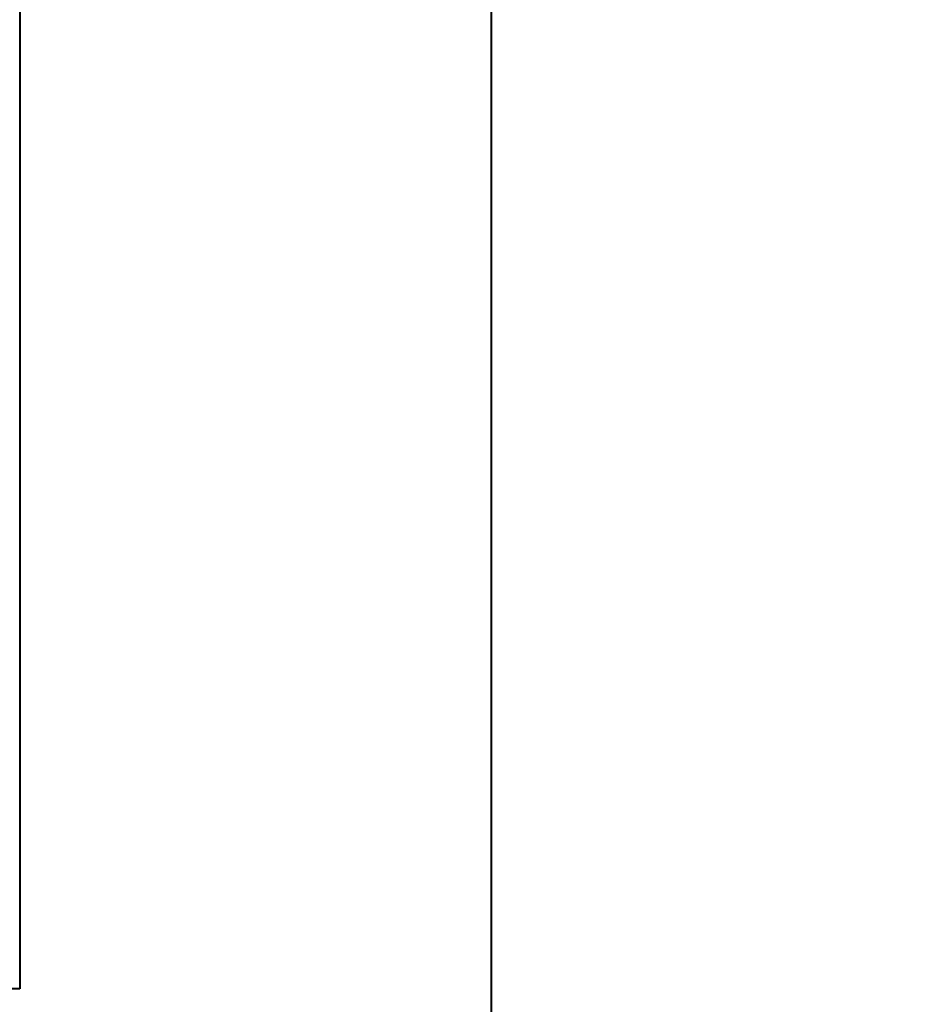
# Model space of a CAD drawing. Units: inches. Extents: x 459864 to 460310, y 324185 to 324787.
# Tile 105 of 112: x 460238 to 460255, y 324292 to 324311. Entities that reach past the tile are written whole.
import ezdxf

# ---------------------------------------------------------------- set-up
doc = ezdxf.new("R2010")
doc.units = ezdxf.units.IN
doc.layers.add('A-ANNO-DIMS', color=2, linetype='Continuous', lineweight=18)
doc.layers.add('A-WALL', color=7, linetype='Continuous', lineweight=40)
doc.styles.get("Standard").update_dxf_attribs({"font": 'arial.ttf'})
doc.dimstyles.new('ISO-25', dxfattribs={"dimtxt": 6, "dimasz": 2.5, "dimexe": 1.25, "dimexo": 0.625, "dimtad": 1, "dimdec": 1, "dimlunit": 3, "dimtxsty": 'Standard', "dimcen": 2.5, "dimadec": 0, "dimazin": 0, "dimtfac": 1, "dimtdec": 1, "dimtmove": 0, "dimatfit": 3, "dimfxl": 1, "dimarcsym": 0})

# ---------------------------------------------------------------- blocks, each defined once
blk = doc.blocks.new('*D21')
at = {"layer": 'A-ANNO-DIMS', "color": 0, "lineweight": -2, "transparency": 16777216}
for p, q in [((460247.74, 324715.483), (460309.58, 324715.483)), ((460308.33, 324712.983), (460308.33, 324285.983)), ((460247.74, 324283.483), (460309.58, 324283.483))]:
    blk.add_line(p, q, dxfattribs=at)
at = {"layer": 'A-ANNO-DIMS', "color": 0, "transparency": 16777216}
for points in [[(460307.914, 324712.983), (460308.747, 324712.983), (460308.33, 324715.483)], [(460307.914, 324285.983), (460308.747, 324285.983), (460308.33, 324283.483)]]:
    blk.add_solid(points, dxfattribs=at)
at = {"layer": 'Defpoints', "color": 0, "transparency": 16777216}
for p in [(460247.115, 324715.483), (460247.115, 324283.483), (460308.33, 324283.483)]:
    blk.add_point(p, dxfattribs=at)
at = {"layer": 'A-ANNO-DIMS', "color": 0, "transparency": 16777216, "insert": (460304.64, 324499.483), "char_height": 6, "attachment_point": 5, "rotation": 90}
blk.add_mtext("36'", dxfattribs=at)
blk = doc.blocks.new('*D62')
at = {"layer": 'A-ANNO-DIMS', "color": 0, "lineweight": -2, "transparency": 16777216}
for p, q in [((460247.74, 324332.739), (460278.765, 324332.739)), ((460277.515, 324330.239), (460277.515, 324285.983)), ((460247.74, 324283.483), (460278.765, 324283.483))]:
    blk.add_line(p, q, dxfattribs=at)
at = {"layer": 'A-ANNO-DIMS', "color": 0, "transparency": 16777216}
for points in [[(460277.098, 324330.239), (460277.932, 324330.239), (460277.515, 324332.739)], [(460277.098, 324285.983), (460277.932, 324285.983), (460277.515, 324283.483)]]:
    blk.add_solid(points, dxfattribs=at)
at = {"layer": 'Defpoints', "color": 0, "transparency": 16777216}
for p in [(460247.115, 324332.739), (460247.115, 324283.483), (460277.515, 324283.483)]:
    blk.add_point(p, dxfattribs=at)
at = {"layer": 'A-ANNO-DIMS', "color": 0, "transparency": 16777216, "insert": (460273.788, 324308.111), "char_height": 6, "attachment_point": 5, "rotation": 90}
blk.add_mtext('4\'-1 1/2"', dxfattribs=at)
blk = doc.blocks.new('*D67')
at = {"layer": 'A-ANNO-DIMS', "color": 0, "lineweight": -2, "transparency": 16777216}
for p, q in [((460208.115, 324284.108), (460208.115, 324315.133)), ((460247.115, 324284.108), (460247.115, 324315.133)), ((460210.615, 324313.883), (460244.615, 324313.883))]:
    blk.add_line(p, q, dxfattribs=at)
at = {"layer": 'A-ANNO-DIMS', "color": 0, "transparency": 16777216}
for points in [[(460210.615, 324314.3), (460210.615, 324313.467), (460208.115, 324313.883)], [(460244.615, 324314.3), (460244.615, 324313.467), (460247.115, 324313.883)]]:
    blk.add_solid(points, dxfattribs=at)
at = {"layer": 'Defpoints', "color": 0, "transparency": 16777216}
for p in [(460247.115, 324313.883), (460208.115, 324283.483), (460247.115, 324283.483)]:
    blk.add_point(p, dxfattribs=at)
at = {"layer": 'A-ANNO-DIMS', "color": 0, "transparency": 16777216, "insert": (460227.615, 324317.574), "char_height": 6, "attachment_point": 5}
blk.add_mtext('3\'-3"', dxfattribs=at)

msp = doc.modelspace()

# ---------------------------------------------------------------- linework, layer by layer
at = {"layer": 'A-WALL'}
for p, q in [((460247.115, 324470.983), (460247.115, 324283.483)), ((460238.115, 324466.483), (460238.115, 324292.483)), ((460238.115, 324292.483), (460088.115, 324292.483))]:
    msp.add_line(p, q, dxfattribs=at)

# ---------------------------------------------------------------- dimensions: what is measured, and where the dimension line sits
at = {"layer": 'A-ANNO-DIMS'}
for base, p1, angle, override, picture, middle in [((460308.33, 324283.483), (460247.115, 324715.483), 90, {"dimclrd": 0, "dimclre": 0, "dimclrt": 0}, '*D21', (460304.64, 324499.483)), ((460277.515, 324283.483), (460247.115, 324332.739), 270, {"dimdec": 1, "dimlfac": 1, "dimrnd": 0, "dimzin": 1, "dimdsep": 46, "dimlunit": 4, "dimfrac": 2}, '*D62', (460273.788, 324308.111))]:
    dim = msp.add_linear_dim(base=base, p1=p1, p2=(460247.115, 324283.483), angle=angle, dimstyle='ISO-25', override=override, dxfattribs=at)
    dim.commit()
    dim.dimension.update_dxf_attribs({"geometry": picture, "text_midpoint": middle})
dim = msp.add_linear_dim(base=(460247.115, 324313.883), p1=(460208.115, 324283.483), p2=(460247.115, 324283.483), dimstyle='ISO-25', override={"dimdec": 1, "dimlfac": 1, "dimrnd": 0, "dimzin": 1, "dimdsep": 46, "dimlunit": 4, "dimfrac": 2}, dxfattribs=at)
dim.commit()
dim.dimension.update_dxf_attribs({"geometry": '*D67', "text_midpoint": (460227.615, 324317.574)})

doc.saveas('drawing.dxf')
